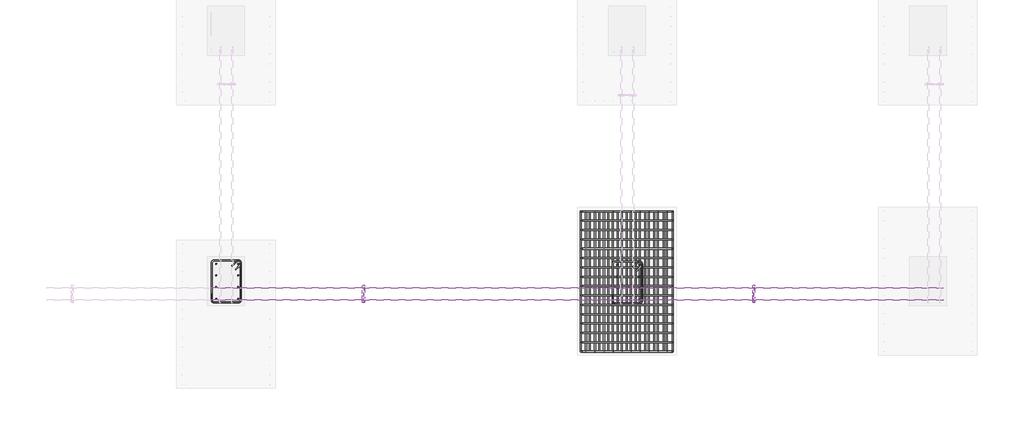
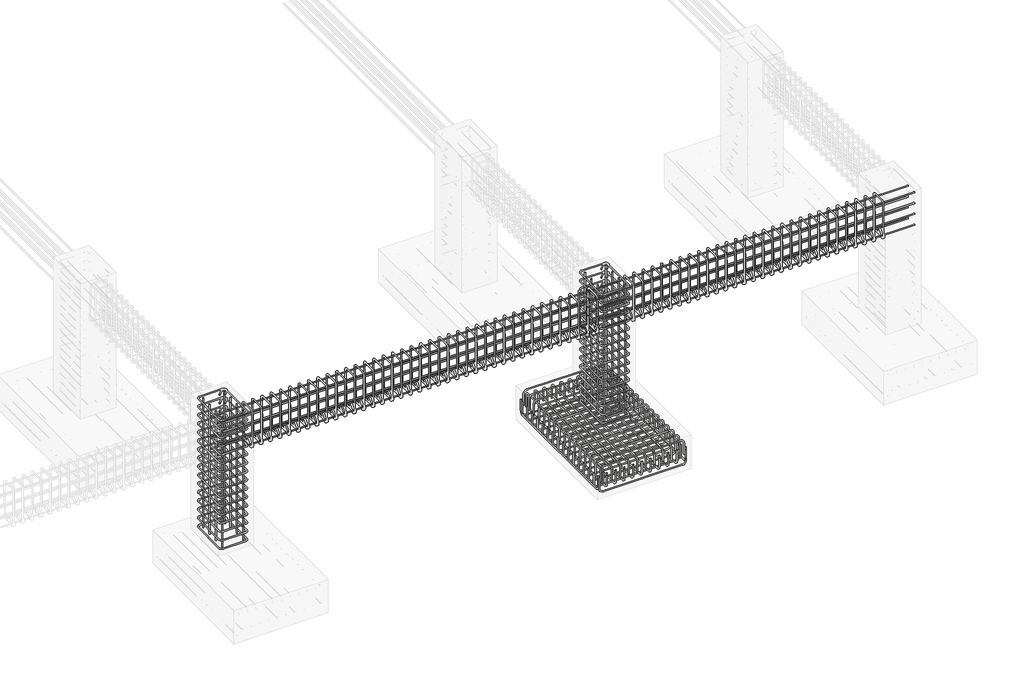
# One storey, part 3 of 16: 16 reinforcing bars.
"""IFC4 building model written with IfcOpenShell, lengths in millimetres."""

from ifc_helpers import new_model, si_unit, point, frame, origin, place, context, project, spatial, polyline, circle_curve, trimmed, segment, composite_curve, source, transform, mapped, element, save
from ifc_brep_helpers import swept_disk

model = new_model("IFC4")

# Units and contexts
model_context = context("Model", 3, world=origin())
ifc_project = project(units=[si_unit("LENGTHUNIT", "METRE", prefix="MILLI")], contexts=[model_context])

# Site, building, storey
site = spatial("IfcSite", under=ifc_project)
building = spatial("IfcBuilding", under=site)
storey = spatial("IfcBuildingStorey", under=building, Elevation=-1828.8)

# Reinforcing bars
placement = place(None, origin())
reinforcing_bar_shape = source(origin(), model_context, "Body", "SolidModel", [
    swept_disk(composite_curve([segment(polyline([(3102.3197974, -311.9348046, -2028.4710597), (3102.3197974, -311.9348046, -2175.7710597)]), True, "CONTINUOUS"), segment(trimmed(circle_curve(frame((3055.9697974, -311.9348046, -2175.7710597), z_axis=(0.0, 1.0, 0.0), x_axis=(46.34999999999991, 0.0, 0.0)), 46.35), [point((3102.3197974, -311.9348046, -2175.7710597))], [point((3055.9697974, -311.9348046, -2222.1210597))], True, "CARTESIAN"), True, "CONTINUOUS"), segment(polyline([(3055.9697974, -311.9348046, -2222.1210597), (2041.3697974, -311.9348046, -2222.1210597)]), True, "CONTINUOUS"), segment(trimmed(circle_curve(frame((2041.3697974, -311.9348046, -2175.7710597), z_axis=(0.0, 1.0, 0.0), x_axis=(0.0, 0.0, -46.34999999999991)), 46.35), [point((2041.3697974, -311.9348046, -2222.1210597))], [point((1995.0197974, -311.9348046, -2175.7710597))], True, "CARTESIAN"), True, "CONTINUOUS"), segment(polyline([(1995.0197974, -311.9348046, -2175.7710597), (1995.0197974, -311.9348046, -2028.4710597)]), True, "CONTINUOUS")], self_intersect=False), 6.35),
])
element("IfcReinforcingBar", 1, at=placement, inside=storey, context=model_context, shape_type="MappedRepresentation", body=[
    mapped(reinforcing_bar_shape, transform((0.0, 0.0, 0.0), x_axis=(1.0, 0.0, 0.0), y_axis=(0.0, 1.0, 0.0), z_axis=(0.0, 0.0, 1.0))),
    mapped(reinforcing_bar_shape, transform((0.0, -113.82, 0.0), x_axis=(1.0, 0.0, 0.0), y_axis=(0.0, 1.0, 0.0), z_axis=(0.0, 0.0, 1.0))),
    mapped(reinforcing_bar_shape, transform((0.0, -227.64, 0.0), x_axis=(1.0, 0.0, 0.0), y_axis=(0.0, 1.0, 0.0), z_axis=(0.0, 0.0, 1.0))),
    mapped(reinforcing_bar_shape, transform((0.0, -341.46, 0.0), x_axis=(1.0, 0.0, 0.0), y_axis=(0.0, 1.0, 0.0), z_axis=(0.0, 0.0, 1.0))),
    mapped(reinforcing_bar_shape, transform((0.0, -455.28, 0.0), x_axis=(1.0, 0.0, 0.0), y_axis=(0.0, 1.0, 0.0), z_axis=(0.0, 0.0, 1.0))),
    mapped(reinforcing_bar_shape, transform((0.0, -569.1, 0.0), x_axis=(1.0, 0.0, 0.0), y_axis=(0.0, 1.0, 0.0), z_axis=(0.0, 0.0, 1.0))),
    mapped(reinforcing_bar_shape, transform((0.0, -682.92, 0.0), x_axis=(1.0, 0.0, 0.0), y_axis=(0.0, 1.0, 0.0), z_axis=(0.0, 0.0, 1.0))),
    mapped(reinforcing_bar_shape, transform((0.0, -796.74, 0.0), x_axis=(1.0, 0.0, 0.0), y_axis=(0.0, 1.0, 0.0), z_axis=(0.0, 0.0, 1.0))),
    mapped(reinforcing_bar_shape, transform((0.0, -910.56, 0.0), x_axis=(1.0, 0.0, 0.0), y_axis=(0.0, 1.0, 0.0), z_axis=(0.0, 0.0, 1.0))),
    mapped(reinforcing_bar_shape, transform((0.0, -1024.38, 0.0), x_axis=(1.0, 0.0, 0.0), y_axis=(0.0, 1.0, 0.0), z_axis=(0.0, 0.0, 1.0))),
    mapped(reinforcing_bar_shape, transform((0.0, -1138.2, 0.0), x_axis=(1.0, 0.0, 0.0), y_axis=(0.0, 1.0, 0.0), z_axis=(0.0, 0.0, 1.0))),
    mapped(reinforcing_bar_shape, transform((0.0, -1252.02, 0.0), x_axis=(1.0, 0.0, 0.0), y_axis=(0.0, 1.0, 0.0), z_axis=(0.0, 0.0, 1.0))),
    mapped(reinforcing_bar_shape, transform((0.0, -1365.84, 0.0), x_axis=(1.0, 0.0, 0.0), y_axis=(0.0, 1.0, 0.0), z_axis=(0.0, 0.0, 1.0))),
    mapped(reinforcing_bar_shape, transform((0.0, -1479.66, 0.0), x_axis=(1.0, 0.0, 0.0), y_axis=(0.0, 1.0, 0.0), z_axis=(0.0, 0.0, 1.0))),
    mapped(reinforcing_bar_shape, transform((0.0, -1593.48, 0.0), x_axis=(1.0, 0.0, 0.0), y_axis=(0.0, 1.0, 0.0), z_axis=(0.0, 0.0, 1.0))),
    mapped(reinforcing_bar_shape, transform((0.0, -1707.3, 0.0), x_axis=(1.0, 0.0, 0.0), y_axis=(0.0, 1.0, 0.0), z_axis=(0.0, 0.0, 1.0))),
])
reinforcing_bar_2_shape = source(origin(), model_context, "Body", "SolidModel", [
    swept_disk(composite_curve([segment(polyline([(2013.4757234, -311.9348046, -2081.4939987), (2013.4757234, -311.9348046, -1934.1939987)]), True, "CONTINUOUS"), segment(trimmed(circle_curve(frame((2059.8257234, -311.9348046, -1934.1939987), z_axis=(0.0, 1.0, 0.0), x_axis=(-46.34999999999968, 0.0, 0.0)), 46.35), [point((2013.4757234, -311.9348046, -1934.1939987))], [point((2059.8257234, -311.9348046, -1887.8439987))], True, "CARTESIAN"), True, "CONTINUOUS"), segment(polyline([(2059.8257234, -311.9348046, -1887.8439987), (3033.5450702, -311.9348046, -1887.8439987)]), True, "CONTINUOUS"), segment(trimmed(circle_curve(frame((3033.5450702, -311.9348046, -1934.1939987), z_axis=(0.0, 1.0, 0.0), x_axis=(0.0, 0.0, 46.350000000000136)), 46.35), [point((3033.5450702, -311.9348046, -1887.8439987))], [point((3079.8950702, -311.9348046, -1934.1939987))], True, "CARTESIAN"), True, "CONTINUOUS"), segment(polyline([(3079.8950702, -311.9348046, -1934.1939987), (3079.8950702, -311.9348046, -2081.4939987)]), True, "CONTINUOUS")], self_intersect=False), 6.35),
])
element("IfcReinforcingBar", 2, at=placement, inside=storey, context=model_context, shape_type="MappedRepresentation", body=[
    mapped(reinforcing_bar_2_shape, transform((0.0, 0.0, 0.0), x_axis=(1.0, 0.0, 0.0), y_axis=(0.0, 1.0, 0.0), z_axis=(0.0, 0.0, 1.0))),
    mapped(reinforcing_bar_2_shape, transform((0.0, -113.82, 0.0), x_axis=(1.0, 0.0, 0.0), y_axis=(0.0, 1.0, 0.0), z_axis=(0.0, 0.0, 1.0))),
    mapped(reinforcing_bar_2_shape, transform((0.0, -227.64, 0.0), x_axis=(1.0, 0.0, 0.0), y_axis=(0.0, 1.0, 0.0), z_axis=(0.0, 0.0, 1.0))),
    mapped(reinforcing_bar_2_shape, transform((0.0, -341.46, 0.0), x_axis=(1.0, 0.0, 0.0), y_axis=(0.0, 1.0, 0.0), z_axis=(0.0, 0.0, 1.0))),
    mapped(reinforcing_bar_2_shape, transform((0.0, -455.28, 0.0), x_axis=(1.0, 0.0, 0.0), y_axis=(0.0, 1.0, 0.0), z_axis=(0.0, 0.0, 1.0))),
    mapped(reinforcing_bar_2_shape, transform((0.0, -569.1, 0.0), x_axis=(1.0, 0.0, 0.0), y_axis=(0.0, 1.0, 0.0), z_axis=(0.0, 0.0, 1.0))),
    mapped(reinforcing_bar_2_shape, transform((0.0, -682.92, 0.0), x_axis=(1.0, 0.0, 0.0), y_axis=(0.0, 1.0, 0.0), z_axis=(0.0, 0.0, 1.0))),
    mapped(reinforcing_bar_2_shape, transform((0.0, -796.74, 0.0), x_axis=(1.0, 0.0, 0.0), y_axis=(0.0, 1.0, 0.0), z_axis=(0.0, 0.0, 1.0))),
    mapped(reinforcing_bar_2_shape, transform((0.0, -910.56, 0.0), x_axis=(1.0, 0.0, 0.0), y_axis=(0.0, 1.0, 0.0), z_axis=(0.0, 0.0, 1.0))),
    mapped(reinforcing_bar_2_shape, transform((0.0, -1024.38, 0.0), x_axis=(1.0, 0.0, 0.0), y_axis=(0.0, 1.0, 0.0), z_axis=(0.0, 0.0, 1.0))),
    mapped(reinforcing_bar_2_shape, transform((0.0, -1138.2, 0.0), x_axis=(1.0, 0.0, 0.0), y_axis=(0.0, 1.0, 0.0), z_axis=(0.0, 0.0, 1.0))),
    mapped(reinforcing_bar_2_shape, transform((0.0, -1252.02, 0.0), x_axis=(1.0, 0.0, 0.0), y_axis=(0.0, 1.0, 0.0), z_axis=(0.0, 0.0, 1.0))),
    mapped(reinforcing_bar_2_shape, transform((0.0, -1365.84, 0.0), x_axis=(1.0, 0.0, 0.0), y_axis=(0.0, 1.0, 0.0), z_axis=(0.0, 0.0, 1.0))),
    mapped(reinforcing_bar_2_shape, transform((0.0, -1479.66, 0.0), x_axis=(1.0, 0.0, 0.0), y_axis=(0.0, 1.0, 0.0), z_axis=(0.0, 0.0, 1.0))),
    mapped(reinforcing_bar_2_shape, transform((0.0, -1593.48, 0.0), x_axis=(1.0, 0.0, 0.0), y_axis=(0.0, 1.0, 0.0), z_axis=(0.0, 0.0, 1.0))),
    mapped(reinforcing_bar_2_shape, transform((0.0, -1707.3, 0.0), x_axis=(1.0, 0.0, 0.0), y_axis=(0.0, 1.0, 0.0), z_axis=(0.0, 0.0, 1.0))),
])
reinforcing_bar_3_shape = source(origin(), model_context, "Body", "SolidModel", [
    swept_disk(composite_curve([segment(polyline([(3029.9434064, -311.9348046, -2112.6585679), (3029.9434064, -311.9348046, -1965.3585679)]), True, "CONTINUOUS"), segment(trimmed(circle_curve(frame((3029.9434064, -358.2848046, -1965.3585679), z_axis=(1.0, 0.0, 0.0), x_axis=(0.0, 46.349999999999966, 0.0)), 46.35), [point((3029.9434064, -311.9348046, -1965.3585679))], [point((3029.9434064, -358.2848046, -1919.0085679))], True, "CARTESIAN"), True, "CONTINUOUS"), segment(polyline([(3029.9434064, -358.2848046, -1919.0085679), (3029.9434064, -1972.8848046, -1919.0085679)]), True, "CONTINUOUS"), segment(trimmed(circle_curve(frame((3029.9434064, -1972.8848046, -1965.3585679), z_axis=(1.0, 0.0, 0.0), x_axis=(0.0, 0.0, 46.350000000000136)), 46.35), [point((3029.9434064, -1972.8848046, -1919.0085679))], [point((3029.9434064, -2019.2348046, -1965.3585679))], True, "CARTESIAN"), True, "CONTINUOUS"), segment(polyline([(3029.9434064, -2019.2348046, -1965.3585679), (3029.9434064, -2019.2348046, -2112.6585679)]), True, "CONTINUOUS")], self_intersect=False), 6.35),
])
element("IfcReinforcingBar", 3, at=placement, inside=storey, context=model_context, shape_type="MappedRepresentation", body=[
    mapped(reinforcing_bar_3_shape, transform((0.0, 0.0, 0.0), x_axis=(1.0, 0.0, 0.0), y_axis=(0.0, 1.0, 0.0), z_axis=(0.0, 0.0, 1.0))),
    mapped(reinforcing_bar_3_shape, transform((-109.2679104, 0.0, 0.0), x_axis=(1.0, 0.0, 0.0), y_axis=(0.0, 1.0, 0.0), z_axis=(0.0, 0.0, 1.0))),
    mapped(reinforcing_bar_3_shape, transform((-218.5358207, 0.0, 0.0), x_axis=(1.0, 0.0, 0.0), y_axis=(0.0, 1.0, 0.0), z_axis=(0.0, 0.0, 1.0))),
    mapped(reinforcing_bar_3_shape, transform((-327.8037311, 0.0, 0.0), x_axis=(1.0, 0.0, 0.0), y_axis=(0.0, 1.0, 0.0), z_axis=(0.0, 0.0, 1.0))),
    mapped(reinforcing_bar_3_shape, transform((-437.0716415, 0.0, 0.0), x_axis=(1.0, 0.0, 0.0), y_axis=(0.0, 1.0, 0.0), z_axis=(0.0, 0.0, 1.0))),
    mapped(reinforcing_bar_3_shape, transform((-546.3395518, 0.0, 0.0), x_axis=(1.0, 0.0, 0.0), y_axis=(0.0, 1.0, 0.0), z_axis=(0.0, 0.0, 1.0))),
    mapped(reinforcing_bar_3_shape, transform((-655.6074622, 0.0, 0.0), x_axis=(1.0, 0.0, 0.0), y_axis=(0.0, 1.0, 0.0), z_axis=(0.0, 0.0, 1.0))),
    mapped(reinforcing_bar_3_shape, transform((-764.8753726, 0.0, 0.0), x_axis=(1.0, 0.0, 0.0), y_axis=(0.0, 1.0, 0.0), z_axis=(0.0, 0.0, 1.0))),
    mapped(reinforcing_bar_3_shape, transform((-874.1432829, 0.0, 0.0), x_axis=(1.0, 0.0, 0.0), y_axis=(0.0, 1.0, 0.0), z_axis=(0.0, 0.0, 1.0))),
    mapped(reinforcing_bar_3_shape, transform((-983.4111933, 0.0, 0.0), x_axis=(1.0, 0.0, 0.0), y_axis=(0.0, 1.0, 0.0), z_axis=(0.0, 0.0, 1.0))),
])
reinforcing_bar_4_shape = source(origin(), model_context, "Body", "SolidModel", [
    swept_disk(composite_curve([segment(polyline([(1981.7657332, -311.9348046, -1996.4434391), (1981.7657332, -311.9348046, -2143.7434391)]), True, "CONTINUOUS"), segment(trimmed(circle_curve(frame((1981.7657332, -358.2848046, -2143.7434391), z_axis=(-1.0, 0.0, 0.0), x_axis=(0.0, 46.349999999999966, 0.0)), 46.35), [point((1981.7657332, -311.9348046, -2143.7434391))], [point((1981.7657332, -358.2848046, -2190.0934391))], True, "CARTESIAN"), True, "CONTINUOUS"), segment(polyline([(1981.7657332, -358.2848046, -2190.0934391), (1981.7657332, -1972.8848046, -2190.0934391)]), True, "CONTINUOUS"), segment(trimmed(circle_curve(frame((1981.7657332, -1972.8848046, -2143.7434391), z_axis=(-1.0, 0.0, 0.0), x_axis=(0.0, 0.0, -46.34999999999991)), 46.35), [point((1981.7657332, -1972.8848046, -2190.0934391))], [point((1981.7657332, -2019.2348046, -2143.7434391))], True, "CARTESIAN"), True, "CONTINUOUS"), segment(polyline([(1981.7657332, -2019.2348046, -2143.7434391), (1981.7657332, -2019.2348046, -1996.4434391)]), True, "CONTINUOUS")], self_intersect=False), 6.35),
])
element("IfcReinforcingBar", 4, at=placement, inside=storey, context=model_context, shape_type="MappedRepresentation", body=[
    mapped(reinforcing_bar_4_shape, transform((0.0, 0.0, 0.0), x_axis=(1.0, 0.0, 0.0), y_axis=(0.0, 1.0, 0.0), z_axis=(0.0, 0.0, 1.0))),
    mapped(reinforcing_bar_4_shape, transform((112.0554064, 0.0, 0.0), x_axis=(1.0, 0.0, 0.0), y_axis=(0.0, 1.0, 0.0), z_axis=(0.0, 0.0, 1.0))),
    mapped(reinforcing_bar_4_shape, transform((224.1108128, 0.0, 0.0), x_axis=(1.0, 0.0, 0.0), y_axis=(0.0, 1.0, 0.0), z_axis=(0.0, 0.0, 1.0))),
    mapped(reinforcing_bar_4_shape, transform((336.1662192, 0.0, 0.0), x_axis=(1.0, 0.0, 0.0), y_axis=(0.0, 1.0, 0.0), z_axis=(0.0, 0.0, 1.0))),
    mapped(reinforcing_bar_4_shape, transform((448.2216256, 0.0, 0.0), x_axis=(1.0, 0.0, 0.0), y_axis=(0.0, 1.0, 0.0), z_axis=(0.0, 0.0, 1.0))),
    mapped(reinforcing_bar_4_shape, transform((560.2770321, 0.0, 0.0), x_axis=(1.0, 0.0, 0.0), y_axis=(0.0, 1.0, 0.0), z_axis=(0.0, 0.0, 1.0))),
    mapped(reinforcing_bar_4_shape, transform((672.3324385, 0.0, 0.0), x_axis=(1.0, 0.0, 0.0), y_axis=(0.0, 1.0, 0.0), z_axis=(0.0, 0.0, 1.0))),
    mapped(reinforcing_bar_4_shape, transform((784.3878449, 0.0, 0.0), x_axis=(1.0, 0.0, 0.0), y_axis=(0.0, 1.0, 0.0), z_axis=(0.0, 0.0, 1.0))),
    mapped(reinforcing_bar_4_shape, transform((896.4432513, 0.0, 0.0), x_axis=(1.0, 0.0, 0.0), y_axis=(0.0, 1.0, 0.0), z_axis=(0.0, 0.0, 1.0))),
    mapped(reinforcing_bar_4_shape, transform((1008.4986577, 0.0, 0.0), x_axis=(1.0, 0.0, 0.0), y_axis=(0.0, 1.0, 0.0), z_axis=(0.0, 0.0, 1.0))),
    mapped(reinforcing_bar_4_shape, transform((1120.5540641, 0.0, 0.0), x_axis=(1.0, 0.0, 0.0), y_axis=(0.0, 1.0, 0.0), z_axis=(0.0, 0.0, 1.0))),
])
reinforcing_bar_5_shape = source(origin(), model_context, "Body", "SolidModel", [
    swept_disk(composite_curve([segment(polyline([(2618.0584368, -988.86057, -46.35), (2673.8019998, -933.117007, -46.35)]), True, "CONTINUOUS"), segment(trimmed(circle_curve(frame((2695.9697974, -955.2848046, -46.35), z_axis=(0.0, 0.0, -1.0), x_axis=(-22.167797600000085, 22.167797600000085, 0.0)), 31.35), [point((2673.8019998, -933.117007, -46.35))], [point((2727.3197974, -955.2848046, -46.35))], True, "CARTESIAN"), True, "CONTINUOUS"), segment(polyline([(2727.3197974, -955.2848046, -46.35), (2727.3197974, -1399.8848046, -46.35)]), True, "CONTINUOUS"), segment(trimmed(circle_curve(frame((2695.9697974, -1399.8848046, -46.35), z_axis=(0.0, 0.0, -1.0), x_axis=(31.34999999999991, 0.0, 0.0)), 31.35), [point((2727.3197974, -1399.8848046, -46.35))], [point((2695.9697974, -1431.2348046, -46.35))], True, "CARTESIAN"), True, "CONTINUOUS"), segment(polyline([(2695.9697974, -1431.2348046, -46.35), (2401.3697974, -1431.2348046, -46.35)]), True, "CONTINUOUS"), segment(trimmed(circle_curve(frame((2401.3697974, -1399.8946239, -45.5654144), z_axis=(0.0, 0.025026655153786343, -0.9996867842138424), x_axis=(0.0, -31.34018070000002, -0.7845855999999998)), 31.35), [point((2401.3697974, -1431.2348046, -46.35))], [point((2370.0197974, -1399.8946239, -45.5654144))], True, "CARTESIAN"), True, "CONTINUOUS"), segment(polyline([(2370.0197974, -1399.8946239, -45.5654144), (2370.0197974, -955.2749853, -34.4345856)]), True, "CONTINUOUS"), segment(trimmed(circle_curve(frame((2401.3697974, -955.2749853, -34.4345856), z_axis=(0.0, 0.025026655153786343, -0.9996867842138424), x_axis=(-31.350000000000364, 0.0, 0.0)), 31.35), [point((2370.0197974, -955.2749853, -34.4345856))], [point((2401.3697974, -923.9348046, -33.65))], True, "CARTESIAN"), True, "CONTINUOUS"), segment(polyline([(2401.3697974, -923.9348046, -33.65), (2695.9697974, -923.9348046, -33.65)]), True, "CONTINUOUS"), segment(trimmed(circle_curve(frame((2695.9697974, -955.2848046, -33.65), z_axis=(0.0, 0.0, -1.0), x_axis=(0.0, 31.350000000000023, 0.0)), 31.35), [point((2695.9697974, -923.9348046, -33.65))], [point((2718.137595, -977.4526022, -33.65))], True, "CARTESIAN"), True, "CONTINUOUS"), segment(polyline([(2718.137595, -977.4526022, -33.65), (2662.394032, -1033.1961652, -33.65)]), True, "CONTINUOUS")], self_intersect=False), 6.35),
])
element("IfcReinforcingBar", 5, at=placement, inside=storey, context=model_context, shape_type="MappedRepresentation", body=[
    mapped(reinforcing_bar_5_shape, transform((0.0, 0.0, 0.0), x_axis=(1.0, 0.0, 0.0), y_axis=(0.0, 1.0, 0.0), z_axis=(0.0, 0.0, 1.0))),
    mapped(reinforcing_bar_5_shape, transform((0.0, 0.0, -115.74), x_axis=(1.0, 0.0, 0.0), y_axis=(0.0, 1.0, 0.0), z_axis=(0.0, 0.0, 1.0))),
    mapped(reinforcing_bar_5_shape, transform((0.0, 0.0, -231.48), x_axis=(1.0, 0.0, 0.0), y_axis=(0.0, 1.0, 0.0), z_axis=(0.0, 0.0, 1.0))),
    mapped(reinforcing_bar_5_shape, transform((0.0, 0.0, -347.22), x_axis=(1.0, 0.0, 0.0), y_axis=(0.0, 1.0, 0.0), z_axis=(0.0, 0.0, 1.0))),
    mapped(reinforcing_bar_5_shape, transform((0.0, 0.0, -462.96), x_axis=(1.0, 0.0, 0.0), y_axis=(0.0, 1.0, 0.0), z_axis=(0.0, 0.0, 1.0))),
    mapped(reinforcing_bar_5_shape, transform((0.0, 0.0, -578.7), x_axis=(1.0, 0.0, 0.0), y_axis=(0.0, 1.0, 0.0), z_axis=(0.0, 0.0, 1.0))),
    mapped(reinforcing_bar_5_shape, transform((0.0, 0.0, -694.44), x_axis=(1.0, 0.0, 0.0), y_axis=(0.0, 1.0, 0.0), z_axis=(0.0, 0.0, 1.0))),
    mapped(reinforcing_bar_5_shape, transform((0.0, 0.0, -810.18), x_axis=(1.0, 0.0, 0.0), y_axis=(0.0, 1.0, 0.0), z_axis=(0.0, 0.0, 1.0))),
    mapped(reinforcing_bar_5_shape, transform((0.0, 0.0, -925.92), x_axis=(1.0, 0.0, 0.0), y_axis=(0.0, 1.0, 0.0), z_axis=(0.0, 0.0, 1.0))),
    mapped(reinforcing_bar_5_shape, transform((0.0, 0.0, -1041.66), x_axis=(1.0, 0.0, 0.0), y_axis=(0.0, 1.0, 0.0), z_axis=(0.0, 0.0, 1.0))),
    mapped(reinforcing_bar_5_shape, transform((0.0, 0.0, -1157.4), x_axis=(1.0, 0.0, 0.0), y_axis=(0.0, 1.0, 0.0), z_axis=(0.0, 0.0, 1.0))),
    mapped(reinforcing_bar_5_shape, transform((0.0, 0.0, -1273.14), x_axis=(1.0, 0.0, 0.0), y_axis=(0.0, 1.0, 0.0), z_axis=(0.0, 0.0, 1.0))),
    mapped(reinforcing_bar_5_shape, transform((0.0, 0.0, -1388.88), x_axis=(1.0, 0.0, 0.0), y_axis=(0.0, 1.0, 0.0), z_axis=(0.0, 0.0, 1.0))),
    mapped(reinforcing_bar_5_shape, transform((0.0, 0.0, -1504.62), x_axis=(1.0, 0.0, 0.0), y_axis=(0.0, 1.0, 0.0), z_axis=(0.0, 0.0, 1.0))),
    mapped(reinforcing_bar_5_shape, transform((0.0, 0.0, -1620.36), x_axis=(1.0, 0.0, 0.0), y_axis=(0.0, 1.0, 0.0), z_axis=(0.0, 0.0, 1.0))),
    mapped(reinforcing_bar_5_shape, transform((0.0, 0.0, -1736.1), x_axis=(1.0, 0.0, 0.0), y_axis=(0.0, 1.0, 0.0), z_axis=(0.0, 0.0, 1.0))),
])
reinforcing_bar_6_shape = source(origin(), model_context, "Body", "SolidModel", [
    swept_disk(composite_curve([segment(polyline([(2692.7822559, -962.0668285, -40.0), (2692.7822559, -962.0668285, -1788.8)]), True, "CONTINUOUS")], self_intersect=False), 6.35),
])
element("IfcReinforcingBar", 6, at=placement, inside=storey, context=model_context, shape_type="MappedRepresentation", body=[
    mapped(reinforcing_bar_6_shape, transform((0.0, 0.0, 0.0), x_axis=(1.0, 0.0, 0.0), y_axis=(0.0, 1.0, 0.0), z_axis=(0.0, 0.0, 1.0))),
    mapped(reinforcing_bar_6_shape, transform((0.0, -141.8865927, 0.0), x_axis=(1.0, 0.0, 0.0), y_axis=(0.0, 1.0, 0.0), z_axis=(0.0, 0.0, 1.0))),
    mapped(reinforcing_bar_6_shape, transform((0.0, -283.7731853, 0.0), x_axis=(1.0, 0.0, 0.0), y_axis=(0.0, 1.0, 0.0), z_axis=(0.0, 0.0, 1.0))),
    mapped(reinforcing_bar_6_shape, transform((0.0, -425.659778, 0.0), x_axis=(1.0, 0.0, 0.0), y_axis=(0.0, 1.0, 0.0), z_axis=(0.0, 0.0, 1.0))),
])
reinforcing_bar_7_shape = source(origin(), model_context, "Body", "SolidModel", [
    swept_disk(composite_curve([segment(polyline([(2424.5573388, -962.0668285, -40.0), (2424.5573388, -962.0668285, -1788.8)]), True, "CONTINUOUS")], self_intersect=False), 6.35),
])
element("IfcReinforcingBar", 7, at=placement, inside=storey, context=model_context, shape_type="MappedRepresentation", body=[
    mapped(reinforcing_bar_7_shape, transform((0.0, 0.0, 0.0), x_axis=(1.0, 0.0, 0.0), y_axis=(0.0, 1.0, 0.0), z_axis=(0.0, 0.0, 1.0))),
    mapped(reinforcing_bar_7_shape, transform((0.0, -141.8865927, 0.0), x_axis=(1.0, 0.0, 0.0), y_axis=(0.0, 1.0, 0.0), z_axis=(0.0, 0.0, 1.0))),
    mapped(reinforcing_bar_7_shape, transform((0.0, -283.7731853, 0.0), x_axis=(1.0, 0.0, 0.0), y_axis=(0.0, 1.0, 0.0), z_axis=(0.0, 0.0, 1.0))),
    mapped(reinforcing_bar_7_shape, transform((0.0, -425.659778, 0.0), x_axis=(1.0, 0.0, 0.0), y_axis=(0.0, 1.0, 0.0), z_axis=(0.0, 0.0, 1.0))),
])
reinforcing_bar_8_shape = source(origin(), model_context, "Body", "SolidModel", [
    swept_disk(composite_curve([segment(polyline([(-2258.7415632, -976.86057, -46.35), (-2202.9980002, -921.117007, -46.35)]), True, "CONTINUOUS"), segment(trimmed(circle_curve(frame((-2180.8302026, -943.2848046, -46.35), z_axis=(0.0, 0.0, -1.0), x_axis=(-22.167797600000085, 22.167797600000085, 0.0)), 31.35), [point((-2202.9980002, -921.117007, -46.35))], [point((-2149.4802026, -943.2848046, -46.35))], True, "CARTESIAN"), True, "CONTINUOUS"), segment(polyline([(-2149.4802026, -943.2848046, -46.35), (-2149.4802026, -1387.8848046, -46.35)]), True, "CONTINUOUS"), segment(trimmed(circle_curve(frame((-2180.8302026, -1387.8848046, -46.35), z_axis=(0.0, 0.0, -1.0), x_axis=(31.34999999999991, 0.0, 0.0)), 31.35), [point((-2149.4802026, -1387.8848046, -46.35))], [point((-2180.8302026, -1419.2348046, -46.35))], True, "CARTESIAN"), True, "CONTINUOUS"), segment(polyline([(-2180.8302026, -1419.2348046, -46.35), (-2475.4302026, -1419.2348046, -46.35)]), True, "CONTINUOUS"), segment(trimmed(circle_curve(frame((-2475.4302026, -1387.8946239, -45.5654144), z_axis=(0.0, 0.025026655153786343, -0.9996867842138424), x_axis=(0.0, -31.34018070000002, -0.7845855999999998)), 31.35), [point((-2475.4302026, -1419.2348046, -46.35))], [point((-2506.7802026, -1387.8946239, -45.5654144))], True, "CARTESIAN"), True, "CONTINUOUS"), segment(polyline([(-2506.7802026, -1387.8946239, -45.5654144), (-2506.7802026, -943.2749853, -34.4345856)]), True, "CONTINUOUS"), segment(trimmed(circle_curve(frame((-2475.4302026, -943.2749853, -34.4345856), z_axis=(0.0, 0.025026655153786343, -0.9996867842138424), x_axis=(-31.34999999999991, 0.0, 0.0)), 31.35), [point((-2506.7802026, -943.2749853, -34.4345856))], [point((-2475.4302026, -911.9348046, -33.65))], True, "CARTESIAN"), True, "CONTINUOUS"), segment(polyline([(-2475.4302026, -911.9348046, -33.65), (-2180.8302026, -911.9348046, -33.65)]), True, "CONTINUOUS"), segment(trimmed(circle_curve(frame((-2180.8302026, -943.2848046, -33.65), z_axis=(0.0, 0.0, -1.0), x_axis=(0.0, 31.350000000000023, 0.0)), 31.35), [point((-2180.8302026, -911.9348046, -33.65))], [point((-2158.662405, -965.4526022, -33.65))], True, "CARTESIAN"), True, "CONTINUOUS"), segment(polyline([(-2158.662405, -965.4526022, -33.65), (-2214.405968, -1021.1961652, -33.65)]), True, "CONTINUOUS")], self_intersect=False), 6.35),
])
element("IfcReinforcingBar", 8, at=placement, inside=storey, context=model_context, shape_type="MappedRepresentation", body=[
    mapped(reinforcing_bar_8_shape, transform((0.0, 0.0, 0.0), x_axis=(1.0, 0.0, 0.0), y_axis=(0.0, 1.0, 0.0), z_axis=(0.0, 0.0, 1.0))),
    mapped(reinforcing_bar_8_shape, transform((0.0, 0.0, -115.74), x_axis=(1.0, 0.0, 0.0), y_axis=(0.0, 1.0, 0.0), z_axis=(0.0, 0.0, 1.0))),
    mapped(reinforcing_bar_8_shape, transform((0.0, 0.0, -231.48), x_axis=(1.0, 0.0, 0.0), y_axis=(0.0, 1.0, 0.0), z_axis=(0.0, 0.0, 1.0))),
    mapped(reinforcing_bar_8_shape, transform((0.0, 0.0, -347.22), x_axis=(1.0, 0.0, 0.0), y_axis=(0.0, 1.0, 0.0), z_axis=(0.0, 0.0, 1.0))),
    mapped(reinforcing_bar_8_shape, transform((0.0, 0.0, -462.96), x_axis=(1.0, 0.0, 0.0), y_axis=(0.0, 1.0, 0.0), z_axis=(0.0, 0.0, 1.0))),
    mapped(reinforcing_bar_8_shape, transform((0.0, 0.0, -578.7), x_axis=(1.0, 0.0, 0.0), y_axis=(0.0, 1.0, 0.0), z_axis=(0.0, 0.0, 1.0))),
    mapped(reinforcing_bar_8_shape, transform((0.0, 0.0, -694.44), x_axis=(1.0, 0.0, 0.0), y_axis=(0.0, 1.0, 0.0), z_axis=(0.0, 0.0, 1.0))),
    mapped(reinforcing_bar_8_shape, transform((0.0, 0.0, -810.18), x_axis=(1.0, 0.0, 0.0), y_axis=(0.0, 1.0, 0.0), z_axis=(0.0, 0.0, 1.0))),
    mapped(reinforcing_bar_8_shape, transform((0.0, 0.0, -925.92), x_axis=(1.0, 0.0, 0.0), y_axis=(0.0, 1.0, 0.0), z_axis=(0.0, 0.0, 1.0))),
    mapped(reinforcing_bar_8_shape, transform((0.0, 0.0, -1041.66), x_axis=(1.0, 0.0, 0.0), y_axis=(0.0, 1.0, 0.0), z_axis=(0.0, 0.0, 1.0))),
    mapped(reinforcing_bar_8_shape, transform((0.0, 0.0, -1157.4), x_axis=(1.0, 0.0, 0.0), y_axis=(0.0, 1.0, 0.0), z_axis=(0.0, 0.0, 1.0))),
    mapped(reinforcing_bar_8_shape, transform((0.0, 0.0, -1273.14), x_axis=(1.0, 0.0, 0.0), y_axis=(0.0, 1.0, 0.0), z_axis=(0.0, 0.0, 1.0))),
    mapped(reinforcing_bar_8_shape, transform((0.0, 0.0, -1388.88), x_axis=(1.0, 0.0, 0.0), y_axis=(0.0, 1.0, 0.0), z_axis=(0.0, 0.0, 1.0))),
    mapped(reinforcing_bar_8_shape, transform((0.0, 0.0, -1504.62), x_axis=(1.0, 0.0, 0.0), y_axis=(0.0, 1.0, 0.0), z_axis=(0.0, 0.0, 1.0))),
    mapped(reinforcing_bar_8_shape, transform((0.0, 0.0, -1620.36), x_axis=(1.0, 0.0, 0.0), y_axis=(0.0, 1.0, 0.0), z_axis=(0.0, 0.0, 1.0))),
    mapped(reinforcing_bar_8_shape, transform((0.0, 0.0, -1736.1), x_axis=(1.0, 0.0, 0.0), y_axis=(0.0, 1.0, 0.0), z_axis=(0.0, 0.0, 1.0))),
])
reinforcing_bar_9_shape = source(origin(), model_context, "Body", "SolidModel", [
    swept_disk(composite_curve([segment(polyline([(-2184.0177441, -950.0668285, -40.0), (-2184.0177441, -950.0668285, -1788.8)]), True, "CONTINUOUS")], self_intersect=False), 6.35),
])
element("IfcReinforcingBar", 9, at=placement, inside=storey, context=model_context, shape_type="MappedRepresentation", body=[
    mapped(reinforcing_bar_9_shape, transform((0.0, 0.0, 0.0), x_axis=(1.0, 0.0, 0.0), y_axis=(0.0, 1.0, 0.0), z_axis=(0.0, 0.0, 1.0))),
    mapped(reinforcing_bar_9_shape, transform((0.0, -141.8865927, 0.0), x_axis=(1.0, 0.0, 0.0), y_axis=(0.0, 1.0, 0.0), z_axis=(0.0, 0.0, 1.0))),
    mapped(reinforcing_bar_9_shape, transform((0.0, -283.7731853, 0.0), x_axis=(1.0, 0.0, 0.0), y_axis=(0.0, 1.0, 0.0), z_axis=(0.0, 0.0, 1.0))),
    mapped(reinforcing_bar_9_shape, transform((0.0, -425.659778, 0.0), x_axis=(1.0, 0.0, 0.0), y_axis=(0.0, 1.0, 0.0), z_axis=(0.0, 0.0, 1.0))),
])
reinforcing_bar_10_shape = source(origin(), model_context, "Body", "SolidModel", [
    swept_disk(composite_curve([segment(polyline([(-2452.2426612, -950.0668285, -40.0), (-2452.2426612, -950.0668285, -1788.8)]), True, "CONTINUOUS")], self_intersect=False), 6.35),
])
element("IfcReinforcingBar", 10, at=placement, inside=storey, context=model_context, shape_type="MappedRepresentation", body=[
    mapped(reinforcing_bar_10_shape, transform((0.0, 0.0, 0.0), x_axis=(1.0, 0.0, 0.0), y_axis=(0.0, 1.0, 0.0), z_axis=(0.0, 0.0, 1.0))),
    mapped(reinforcing_bar_10_shape, transform((0.0, -141.8865927, 0.0), x_axis=(1.0, 0.0, 0.0), y_axis=(0.0, 1.0, 0.0), z_axis=(0.0, 0.0, 1.0))),
    mapped(reinforcing_bar_10_shape, transform((0.0, -283.7731853, 0.0), x_axis=(1.0, 0.0, 0.0), y_axis=(0.0, 1.0, 0.0), z_axis=(0.0, 0.0, 1.0))),
    mapped(reinforcing_bar_10_shape, transform((0.0, -425.659778, 0.0), x_axis=(1.0, 0.0, 0.0), y_axis=(0.0, 1.0, 0.0), z_axis=(0.0, 0.0, 1.0))),
])
reinforcing_bar_11_shape = source(origin(), model_context, "Body", "SolidModel", [
    swept_disk(composite_curve([segment(polyline([(5974.9197974, -1309.9734441, -488.7242346), (5974.9197974, -1365.717007, -544.4677976)]), True, "CONTINUOUS"), segment(trimmed(circle_curve(frame((5974.9197974, -1387.8848046, -522.3), z_axis=(-1.0, 0.0, 0.0), x_axis=(0.0, 22.167797600000085, -22.167797600000085)), 31.35), [point((5974.9197974, -1365.717007, -544.4677976))], [point((5974.9197974, -1419.2348046, -522.3))], True, "CARTESIAN"), True, "CONTINUOUS"), segment(polyline([(5974.9197974, -1419.2348046, -522.3), (5974.9197974, -1419.2348046, -77.7)]), True, "CONTINUOUS"), segment(trimmed(circle_curve(frame((5974.9197974, -1387.8848046, -77.7), z_axis=(-1.0, 0.0, 0.0), x_axis=(0.0, -31.34999999999991, 0.0)), 31.35), [point((5974.9197974, -1419.2348046, -77.7))], [point((5974.9197974, -1387.8848046, -46.35))], True, "CARTESIAN"), True, "CONTINUOUS"), segment(polyline([(5974.9197974, -1387.8848046, -46.35), (5974.9197974, -1243.2848046, -46.35)]), True, "CONTINUOUS"), segment(trimmed(circle_curve(frame((5975.704383, -1243.2848046, -77.6901807), z_axis=(-0.9996867842138424, 0.0, -0.025026655153786322), x_axis=(-0.784585600000355, 0.0, 31.340180699999998)), 31.35), [point((5974.9197974, -1243.2848046, -46.35))], [point((5975.704383, -1211.9348046, -77.6901807))], True, "CARTESIAN"), True, "CONTINUOUS"), segment(polyline([(5975.704383, -1211.9348046, -77.6901807), (5986.8352117, -1211.9348046, -522.3098193)]), True, "CONTINUOUS"), segment(trimmed(circle_curve(frame((5986.8352117, -1243.2848046, -522.3098193), z_axis=(-0.9996867842138424, 0.0, -0.025026655153786322), x_axis=(0.0, 31.34999999999991, 0.0)), 31.35), [point((5986.8352117, -1211.9348046, -522.3098193))], [point((5987.6197974, -1243.2848046, -553.65))], True, "CARTESIAN"), True, "CONTINUOUS"), segment(polyline([(5987.6197974, -1243.2848046, -553.65), (5987.6197974, -1387.8848046, -553.65)]), True, "CONTINUOUS"), segment(trimmed(circle_curve(frame((5987.6197974, -1387.8848046, -522.3), z_axis=(-1.0, 0.0, 0.0), x_axis=(0.0, 0.0, -31.350000000000023)), 31.35), [point((5987.6197974, -1387.8848046, -553.65))], [point((5987.6197974, -1410.0526022, -500.1322024))], True, "CARTESIAN"), True, "CONTINUOUS"), segment(polyline([(5987.6197974, -1410.0526022, -500.1322024), (5987.6197974, -1354.3090393, -444.3886395)]), True, "CONTINUOUS")], self_intersect=False), 6.35),
])
element("IfcReinforcingBar", 11, at=placement, inside=storey, context=model_context, shape_type="MappedRepresentation", body=[
    mapped(reinforcing_bar_11_shape, transform((0.0, 0.0, 0.0), x_axis=(1.0, 0.0, 0.0), y_axis=(0.0, 1.0, 0.0), z_axis=(0.0, 0.0, 1.0))),
    mapped(reinforcing_bar_11_shape, transform((-118.3296297, 0.0, 0.0), x_axis=(1.0, 0.0, 0.0), y_axis=(0.0, 1.0, 0.0), z_axis=(0.0, 0.0, 1.0))),
    mapped(reinforcing_bar_11_shape, transform((-236.6592593, 0.0, 0.0), x_axis=(1.0, 0.0, 0.0), y_axis=(0.0, 1.0, 0.0), z_axis=(0.0, 0.0, 1.0))),
    mapped(reinforcing_bar_11_shape, transform((-354.988889, 0.0, 0.0), x_axis=(1.0, 0.0, 0.0), y_axis=(0.0, 1.0, 0.0), z_axis=(0.0, 0.0, 1.0))),
    mapped(reinforcing_bar_11_shape, transform((-473.3185186, 0.0, 0.0), x_axis=(1.0, 0.0, 0.0), y_axis=(0.0, 1.0, 0.0), z_axis=(0.0, 0.0, 1.0))),
    mapped(reinforcing_bar_11_shape, transform((-591.6481483, 0.0, 0.0), x_axis=(1.0, 0.0, 0.0), y_axis=(0.0, 1.0, 0.0), z_axis=(0.0, 0.0, 1.0))),
    mapped(reinforcing_bar_11_shape, transform((-709.9777779, 0.0, 0.0), x_axis=(1.0, 0.0, 0.0), y_axis=(0.0, 1.0, 0.0), z_axis=(0.0, 0.0, 1.0))),
    mapped(reinforcing_bar_11_shape, transform((-828.3074076, 0.0, 0.0), x_axis=(1.0, 0.0, 0.0), y_axis=(0.0, 1.0, 0.0), z_axis=(0.0, 0.0, 1.0))),
    mapped(reinforcing_bar_11_shape, transform((-946.6370372, 0.0, 0.0), x_axis=(1.0, 0.0, 0.0), y_axis=(0.0, 1.0, 0.0), z_axis=(0.0, 0.0, 1.0))),
    mapped(reinforcing_bar_11_shape, transform((-1064.9666669, 0.0, 0.0), x_axis=(1.0, 0.0, 0.0), y_axis=(0.0, 1.0, 0.0), z_axis=(0.0, 0.0, 1.0))),
    mapped(reinforcing_bar_11_shape, transform((-1183.2962965, 0.0, 0.0), x_axis=(1.0, 0.0, 0.0), y_axis=(0.0, 1.0, 0.0), z_axis=(0.0, 0.0, 1.0))),
    mapped(reinforcing_bar_11_shape, transform((-1301.6259262, 0.0, 0.0), x_axis=(1.0, 0.0, 0.0), y_axis=(0.0, 1.0, 0.0), z_axis=(0.0, 0.0, 1.0))),
    mapped(reinforcing_bar_11_shape, transform((-1419.9555558, 0.0, 0.0), x_axis=(1.0, 0.0, 0.0), y_axis=(0.0, 1.0, 0.0), z_axis=(0.0, 0.0, 1.0))),
    mapped(reinforcing_bar_11_shape, transform((-1538.2851855, 0.0, 0.0), x_axis=(1.0, 0.0, 0.0), y_axis=(0.0, 1.0, 0.0), z_axis=(0.0, 0.0, 1.0))),
    mapped(reinforcing_bar_11_shape, transform((-1656.6148151, 0.0, 0.0), x_axis=(1.0, 0.0, 0.0), y_axis=(0.0, 1.0, 0.0), z_axis=(0.0, 0.0, 1.0))),
    mapped(reinforcing_bar_11_shape, transform((-1774.9444448, 0.0, 0.0), x_axis=(1.0, 0.0, 0.0), y_axis=(0.0, 1.0, 0.0), z_axis=(0.0, 0.0, 1.0))),
    mapped(reinforcing_bar_11_shape, transform((-1893.2740744, 0.0, 0.0), x_axis=(1.0, 0.0, 0.0), y_axis=(0.0, 1.0, 0.0), z_axis=(0.0, 0.0, 1.0))),
    mapped(reinforcing_bar_11_shape, transform((-2011.6037041, 0.0, 0.0), x_axis=(1.0, 0.0, 0.0), y_axis=(0.0, 1.0, 0.0), z_axis=(0.0, 0.0, 1.0))),
    mapped(reinforcing_bar_11_shape, transform((-2129.9333337, 0.0, 0.0), x_axis=(1.0, 0.0, 0.0), y_axis=(0.0, 1.0, 0.0), z_axis=(0.0, 0.0, 1.0))),
    mapped(reinforcing_bar_11_shape, transform((-2248.2629634, 0.0, 0.0), x_axis=(1.0, 0.0, 0.0), y_axis=(0.0, 1.0, 0.0), z_axis=(0.0, 0.0, 1.0))),
    mapped(reinforcing_bar_11_shape, transform((-2366.592593, 0.0, 0.0), x_axis=(1.0, 0.0, 0.0), y_axis=(0.0, 1.0, 0.0), z_axis=(0.0, 0.0, 1.0))),
    mapped(reinforcing_bar_11_shape, transform((-2484.9222227, 0.0, 0.0), x_axis=(1.0, 0.0, 0.0), y_axis=(0.0, 1.0, 0.0), z_axis=(0.0, 0.0, 1.0))),
    mapped(reinforcing_bar_11_shape, transform((-2603.2518523, 0.0, 0.0), x_axis=(1.0, 0.0, 0.0), y_axis=(0.0, 1.0, 0.0), z_axis=(0.0, 0.0, 1.0))),
    mapped(reinforcing_bar_11_shape, transform((-2721.581482, 0.0, 0.0), x_axis=(1.0, 0.0, 0.0), y_axis=(0.0, 1.0, 0.0), z_axis=(0.0, 0.0, 1.0))),
    mapped(reinforcing_bar_11_shape, transform((-2839.9111117, 0.0, 0.0), x_axis=(1.0, 0.0, 0.0), y_axis=(0.0, 1.0, 0.0), z_axis=(0.0, 0.0, 1.0))),
    mapped(reinforcing_bar_11_shape, transform((-2958.2407413, 0.0, 0.0), x_axis=(1.0, 0.0, 0.0), y_axis=(0.0, 1.0, 0.0), z_axis=(0.0, 0.0, 1.0))),
    mapped(reinforcing_bar_11_shape, transform((-3076.570371, 0.0, 0.0), x_axis=(1.0, 0.0, 0.0), y_axis=(0.0, 1.0, 0.0), z_axis=(0.0, 0.0, 1.0))),
    mapped(reinforcing_bar_11_shape, transform((-3194.9000006, 0.0, 0.0), x_axis=(1.0, 0.0, 0.0), y_axis=(0.0, 1.0, 0.0), z_axis=(0.0, 0.0, 1.0))),
])
reinforcing_bar_12_shape = source(origin(), model_context, "Body", "SolidModel", [
    swept_disk(composite_curve([segment(polyline([(6391.2697974, -1387.8848046, -524.4645649), (2363.6697974, -1387.8848046, -524.4645649)]), True, "CONTINUOUS")], self_intersect=False), 6.35),
])
element("IfcReinforcingBar", 12, at=placement, inside=storey, context=model_context, shape_type="MappedRepresentation", body=[
    mapped(reinforcing_bar_12_shape, transform((0.0, 0.0, 0.0), x_axis=(1.0, 0.0, 0.0), y_axis=(0.0, 1.0, 0.0), z_axis=(0.0, 0.0, 1.0))),
    mapped(reinforcing_bar_12_shape, transform((0.0, 0.0, 146.3763852), x_axis=(1.0, 0.0, 0.0), y_axis=(0.0, 1.0, 0.0), z_axis=(0.0, 0.0, 1.0))),
    mapped(reinforcing_bar_12_shape, transform((0.0, 0.0, 292.7527704), x_axis=(1.0, 0.0, 0.0), y_axis=(0.0, 1.0, 0.0), z_axis=(0.0, 0.0, 1.0))),
    mapped(reinforcing_bar_12_shape, transform((0.0, 0.0, 439.1291556), x_axis=(1.0, 0.0, 0.0), y_axis=(0.0, 1.0, 0.0), z_axis=(0.0, 0.0, 1.0))),
])
reinforcing_bar_13_shape = source(origin(), model_context, "Body", "SolidModel", [
    swept_disk(composite_curve([segment(polyline([(6391.2697974, -1243.2848046, -524.4645649), (2363.6697974, -1243.2848046, -524.4645649)]), True, "CONTINUOUS")], self_intersect=False), 6.35),
])
element("IfcReinforcingBar", 13, at=placement, inside=storey, context=model_context, shape_type="MappedRepresentation", body=[
    mapped(reinforcing_bar_13_shape, transform((0.0, 0.0, 0.0), x_axis=(1.0, 0.0, 0.0), y_axis=(0.0, 1.0, 0.0), z_axis=(0.0, 0.0, 1.0))),
    mapped(reinforcing_bar_13_shape, transform((0.0, 0.0, 146.3763852), x_axis=(1.0, 0.0, 0.0), y_axis=(0.0, 1.0, 0.0), z_axis=(0.0, 0.0, 1.0))),
    mapped(reinforcing_bar_13_shape, transform((0.0, 0.0, 292.7527704), x_axis=(1.0, 0.0, 0.0), y_axis=(0.0, 1.0, 0.0), z_axis=(0.0, 0.0, 1.0))),
    mapped(reinforcing_bar_13_shape, transform((0.0, 0.0, 439.1291556), x_axis=(1.0, 0.0, 0.0), y_axis=(0.0, 1.0, 0.0), z_axis=(0.0, 0.0, 1.0))),
])
reinforcing_bar_14_shape = source(origin(), model_context, "Body", "SolidModel", [
    swept_disk(composite_curve([segment(polyline([(2317.3197974, -1309.9734441, -488.7242346), (2317.3197974, -1365.717007, -544.4677976)]), True, "CONTINUOUS"), segment(trimmed(circle_curve(frame((2317.3197974, -1387.8848046, -522.3), z_axis=(-1.0, 0.0, 0.0), x_axis=(0.0, 22.167797600000085, -22.167797600000085)), 31.35), [point((2317.3197974, -1365.717007, -544.4677976))], [point((2317.3197974, -1419.2348046, -522.3))], True, "CARTESIAN"), True, "CONTINUOUS"), segment(polyline([(2317.3197974, -1419.2348046, -522.3), (2317.3197974, -1419.2348046, -77.7)]), True, "CONTINUOUS"), segment(trimmed(circle_curve(frame((2317.3197974, -1387.8848046, -77.7), z_axis=(-1.0, 0.0, 0.0), x_axis=(0.0, -31.34999999999991, 0.0)), 31.35), [point((2317.3197974, -1419.2348046, -77.7))], [point((2317.3197974, -1387.8848046, -46.35))], True, "CARTESIAN"), True, "CONTINUOUS"), segment(polyline([(2317.3197974, -1387.8848046, -46.35), (2317.3197974, -1243.2848046, -46.35)]), True, "CONTINUOUS"), segment(trimmed(circle_curve(frame((2318.104383, -1243.2848046, -77.6901807), z_axis=(-0.9996867842138424, 0.0, -0.025026655153786322), x_axis=(-0.7845855999999003, 0.0, 31.340180699999998)), 31.35), [point((2317.3197974, -1243.2848046, -46.35))], [point((2318.104383, -1211.9348046, -77.6901807))], True, "CARTESIAN"), True, "CONTINUOUS"), segment(polyline([(2318.104383, -1211.9348046, -77.6901807), (2329.2352117, -1211.9348046, -522.3098193)]), True, "CONTINUOUS"), segment(trimmed(circle_curve(frame((2329.2352117, -1243.2848046, -522.3098193), z_axis=(-0.9996867842138424, 0.0, -0.025026655153786322), x_axis=(0.0, 31.34999999999991, 0.0)), 31.35), [point((2329.2352117, -1211.9348046, -522.3098193))], [point((2330.0197974, -1243.2848046, -553.65))], True, "CARTESIAN"), True, "CONTINUOUS"), segment(polyline([(2330.0197974, -1243.2848046, -553.65), (2330.0197974, -1387.8848046, -553.65)]), True, "CONTINUOUS"), segment(trimmed(circle_curve(frame((2330.0197974, -1387.8848046, -522.3), z_axis=(-1.0, 0.0, 0.0), x_axis=(0.0, 0.0, -31.350000000000023)), 31.35), [point((2330.0197974, -1387.8848046, -553.65))], [point((2330.0197974, -1410.0526022, -500.1322024))], True, "CARTESIAN"), True, "CONTINUOUS"), segment(polyline([(2330.0197974, -1410.0526022, -500.1322024), (2330.0197974, -1354.3090393, -444.3886395)]), True, "CONTINUOUS")], self_intersect=False), 6.35),
])
element("IfcReinforcingBar", 14, at=placement, inside=storey, context=model_context, shape_type="MappedRepresentation", body=[
    mapped(reinforcing_bar_14_shape, transform((0.0, 0.0, 0.0), x_axis=(1.0, 0.0, 0.0), y_axis=(0.0, 1.0, 0.0), z_axis=(0.0, 0.0, 1.0))),
    mapped(reinforcing_bar_14_shape, transform((-119.3, 0.0, 0.0), x_axis=(1.0, 0.0, 0.0), y_axis=(0.0, 1.0, 0.0), z_axis=(0.0, 0.0, 1.0))),
    mapped(reinforcing_bar_14_shape, transform((-238.6, 0.0, 0.0), x_axis=(1.0, 0.0, 0.0), y_axis=(0.0, 1.0, 0.0), z_axis=(0.0, 0.0, 1.0))),
    mapped(reinforcing_bar_14_shape, transform((-357.9, 0.0, 0.0), x_axis=(1.0, 0.0, 0.0), y_axis=(0.0, 1.0, 0.0), z_axis=(0.0, 0.0, 1.0))),
    mapped(reinforcing_bar_14_shape, transform((-477.2000001, 0.0, 0.0), x_axis=(1.0, 0.0, 0.0), y_axis=(0.0, 1.0, 0.0), z_axis=(0.0, 0.0, 1.0))),
    mapped(reinforcing_bar_14_shape, transform((-596.5000001, 0.0, 0.0), x_axis=(1.0, 0.0, 0.0), y_axis=(0.0, 1.0, 0.0), z_axis=(0.0, 0.0, 1.0))),
    mapped(reinforcing_bar_14_shape, transform((-715.8000001, 0.0, 0.0), x_axis=(1.0, 0.0, 0.0), y_axis=(0.0, 1.0, 0.0), z_axis=(0.0, 0.0, 1.0))),
    mapped(reinforcing_bar_14_shape, transform((-835.1000001, 0.0, 0.0), x_axis=(1.0, 0.0, 0.0), y_axis=(0.0, 1.0, 0.0), z_axis=(0.0, 0.0, 1.0))),
    mapped(reinforcing_bar_14_shape, transform((-954.4000001, 0.0, 0.0), x_axis=(1.0, 0.0, 0.0), y_axis=(0.0, 1.0, 0.0), z_axis=(0.0, 0.0, 1.0))),
    mapped(reinforcing_bar_14_shape, transform((-1073.7000001, 0.0, 0.0), x_axis=(1.0, 0.0, 0.0), y_axis=(0.0, 1.0, 0.0), z_axis=(0.0, 0.0, 1.0))),
    mapped(reinforcing_bar_14_shape, transform((-1193.0000002, 0.0, 0.0), x_axis=(1.0, 0.0, 0.0), y_axis=(0.0, 1.0, 0.0), z_axis=(0.0, 0.0, 1.0))),
    mapped(reinforcing_bar_14_shape, transform((-1312.3000002, 0.0, 0.0), x_axis=(1.0, 0.0, 0.0), y_axis=(0.0, 1.0, 0.0), z_axis=(0.0, 0.0, 1.0))),
    mapped(reinforcing_bar_14_shape, transform((-1431.6000002, 0.0, 0.0), x_axis=(1.0, 0.0, 0.0), y_axis=(0.0, 1.0, 0.0), z_axis=(0.0, 0.0, 1.0))),
    mapped(reinforcing_bar_14_shape, transform((-1550.9000002, 0.0, 0.0), x_axis=(1.0, 0.0, 0.0), y_axis=(0.0, 1.0, 0.0), z_axis=(0.0, 0.0, 1.0))),
    mapped(reinforcing_bar_14_shape, transform((-1670.2000002, 0.0, 0.0), x_axis=(1.0, 0.0, 0.0), y_axis=(0.0, 1.0, 0.0), z_axis=(0.0, 0.0, 1.0))),
    mapped(reinforcing_bar_14_shape, transform((-1789.5000002, 0.0, 0.0), x_axis=(1.0, 0.0, 0.0), y_axis=(0.0, 1.0, 0.0), z_axis=(0.0, 0.0, 1.0))),
    mapped(reinforcing_bar_14_shape, transform((-1908.8000003, 0.0, 0.0), x_axis=(1.0, 0.0, 0.0), y_axis=(0.0, 1.0, 0.0), z_axis=(0.0, 0.0, 1.0))),
    mapped(reinforcing_bar_14_shape, transform((-2028.1000003, 0.0, 0.0), x_axis=(1.0, 0.0, 0.0), y_axis=(0.0, 1.0, 0.0), z_axis=(0.0, 0.0, 1.0))),
    mapped(reinforcing_bar_14_shape, transform((-2147.4000003, 0.0, 0.0), x_axis=(1.0, 0.0, 0.0), y_axis=(0.0, 1.0, 0.0), z_axis=(0.0, 0.0, 1.0))),
    mapped(reinforcing_bar_14_shape, transform((-2266.7000003, 0.0, 0.0), x_axis=(1.0, 0.0, 0.0), y_axis=(0.0, 1.0, 0.0), z_axis=(0.0, 0.0, 1.0))),
    mapped(reinforcing_bar_14_shape, transform((-2386.0000003, 0.0, 0.0), x_axis=(1.0, 0.0, 0.0), y_axis=(0.0, 1.0, 0.0), z_axis=(0.0, 0.0, 1.0))),
    mapped(reinforcing_bar_14_shape, transform((-2505.3000003, 0.0, 0.0), x_axis=(1.0, 0.0, 0.0), y_axis=(0.0, 1.0, 0.0), z_axis=(0.0, 0.0, 1.0))),
    mapped(reinforcing_bar_14_shape, transform((-2624.6000004, 0.0, 0.0), x_axis=(1.0, 0.0, 0.0), y_axis=(0.0, 1.0, 0.0), z_axis=(0.0, 0.0, 1.0))),
    mapped(reinforcing_bar_14_shape, transform((-2743.9000004, 0.0, 0.0), x_axis=(1.0, 0.0, 0.0), y_axis=(0.0, 1.0, 0.0), z_axis=(0.0, 0.0, 1.0))),
    mapped(reinforcing_bar_14_shape, transform((-2863.2000004, 0.0, 0.0), x_axis=(1.0, 0.0, 0.0), y_axis=(0.0, 1.0, 0.0), z_axis=(0.0, 0.0, 1.0))),
    mapped(reinforcing_bar_14_shape, transform((-2982.5000004, 0.0, 0.0), x_axis=(1.0, 0.0, 0.0), y_axis=(0.0, 1.0, 0.0), z_axis=(0.0, 0.0, 1.0))),
    mapped(reinforcing_bar_14_shape, transform((-3101.8000004, 0.0, 0.0), x_axis=(1.0, 0.0, 0.0), y_axis=(0.0, 1.0, 0.0), z_axis=(0.0, 0.0, 1.0))),
    mapped(reinforcing_bar_14_shape, transform((-3221.1000004, 0.0, 0.0), x_axis=(1.0, 0.0, 0.0), y_axis=(0.0, 1.0, 0.0), z_axis=(0.0, 0.0, 1.0))),
    mapped(reinforcing_bar_14_shape, transform((-3340.4000005, 0.0, 0.0), x_axis=(1.0, 0.0, 0.0), y_axis=(0.0, 1.0, 0.0), z_axis=(0.0, 0.0, 1.0))),
    mapped(reinforcing_bar_14_shape, transform((-3459.7000005, 0.0, 0.0), x_axis=(1.0, 0.0, 0.0), y_axis=(0.0, 1.0, 0.0), z_axis=(0.0, 0.0, 1.0))),
    mapped(reinforcing_bar_14_shape, transform((-3579.0000005, 0.0, 0.0), x_axis=(1.0, 0.0, 0.0), y_axis=(0.0, 1.0, 0.0), z_axis=(0.0, 0.0, 1.0))),
    mapped(reinforcing_bar_14_shape, transform((-3698.3000005, 0.0, 0.0), x_axis=(1.0, 0.0, 0.0), y_axis=(0.0, 1.0, 0.0), z_axis=(0.0, 0.0, 1.0))),
    mapped(reinforcing_bar_14_shape, transform((-3817.6000005, 0.0, 0.0), x_axis=(1.0, 0.0, 0.0), y_axis=(0.0, 1.0, 0.0), z_axis=(0.0, 0.0, 1.0))),
    mapped(reinforcing_bar_14_shape, transform((-3936.9000005, 0.0, 0.0), x_axis=(1.0, 0.0, 0.0), y_axis=(0.0, 1.0, 0.0), z_axis=(0.0, 0.0, 1.0))),
    mapped(reinforcing_bar_14_shape, transform((-4056.2000006, 0.0, 0.0), x_axis=(1.0, 0.0, 0.0), y_axis=(0.0, 1.0, 0.0), z_axis=(0.0, 0.0, 1.0))),
    mapped(reinforcing_bar_14_shape, transform((-4175.5000006, 0.0, 0.0), x_axis=(1.0, 0.0, 0.0), y_axis=(0.0, 1.0, 0.0), z_axis=(0.0, 0.0, 1.0))),
    mapped(reinforcing_bar_14_shape, transform((-4294.8000006, 0.0, 0.0), x_axis=(1.0, 0.0, 0.0), y_axis=(0.0, 1.0, 0.0), z_axis=(0.0, 0.0, 1.0))),
    mapped(reinforcing_bar_14_shape, transform((-4414.1000006, 0.0, 0.0), x_axis=(1.0, 0.0, 0.0), y_axis=(0.0, 1.0, 0.0), z_axis=(0.0, 0.0, 1.0))),
])
reinforcing_bar_15_shape = source(origin(), model_context, "Body", "SolidModel", [
    swept_disk(composite_curve([segment(polyline([(2733.6697974, -1387.8848046, -524.4645649), (-2513.1302026, -1387.8848046, -524.4645649)]), True, "CONTINUOUS")], self_intersect=False), 6.35),
])
element("IfcReinforcingBar", 15, at=placement, inside=storey, context=model_context, shape_type="MappedRepresentation", body=[
    mapped(reinforcing_bar_15_shape, transform((0.0, 0.0, 0.0), x_axis=(1.0, 0.0, 0.0), y_axis=(0.0, 1.0, 0.0), z_axis=(0.0, 0.0, 1.0))),
    mapped(reinforcing_bar_15_shape, transform((0.0, 0.0, 146.3763852), x_axis=(1.0, 0.0, 0.0), y_axis=(0.0, 1.0, 0.0), z_axis=(0.0, 0.0, 1.0))),
    mapped(reinforcing_bar_15_shape, transform((0.0, 0.0, 292.7527704), x_axis=(1.0, 0.0, 0.0), y_axis=(0.0, 1.0, 0.0), z_axis=(0.0, 0.0, 1.0))),
    mapped(reinforcing_bar_15_shape, transform((0.0, 0.0, 439.1291556), x_axis=(1.0, 0.0, 0.0), y_axis=(0.0, 1.0, 0.0), z_axis=(0.0, 0.0, 1.0))),
])
reinforcing_bar_16_shape = source(origin(), model_context, "Body", "SolidModel", [
    swept_disk(composite_curve([segment(polyline([(2733.6697974, -1243.2848046, -524.4645649), (-2513.1302026, -1243.2848046, -524.4645649)]), True, "CONTINUOUS")], self_intersect=False), 6.35),
])
element("IfcReinforcingBar", 16, at=placement, inside=storey, context=model_context, shape_type="MappedRepresentation", body=[
    mapped(reinforcing_bar_16_shape, transform((0.0, 0.0, 0.0), x_axis=(1.0, 0.0, 0.0), y_axis=(0.0, 1.0, 0.0), z_axis=(0.0, 0.0, 1.0))),
    mapped(reinforcing_bar_16_shape, transform((0.0, 0.0, 146.3763852), x_axis=(1.0, 0.0, 0.0), y_axis=(0.0, 1.0, 0.0), z_axis=(0.0, 0.0, 1.0))),
    mapped(reinforcing_bar_16_shape, transform((0.0, 0.0, 292.7527704), x_axis=(1.0, 0.0, 0.0), y_axis=(0.0, 1.0, 0.0), z_axis=(0.0, 0.0, 1.0))),
    mapped(reinforcing_bar_16_shape, transform((0.0, 0.0, 439.1291556), x_axis=(1.0, 0.0, 0.0), y_axis=(0.0, 1.0, 0.0), z_axis=(0.0, 0.0, 1.0))),
])

save(model, "model.ifc")

# Revit data of these elements
# Elements 1, 2, 3, 4, 5, 6, 7, 8, 9, 10, 11, 12, 13, 14, 15, 16 (IfcReinforcingBar)
#   Phase Created = New Construction
